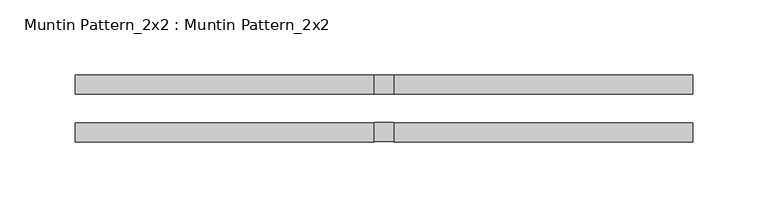
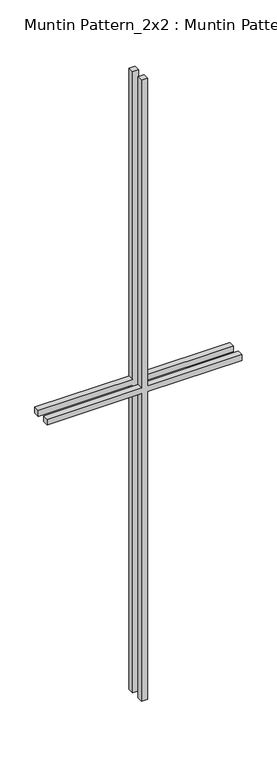
"""IFC4 building model written with IfcOpenShell, lengths in millimetres: proxy geometry, Muntin Pattern_2x2 : Muntin Pattern_2x2."""

from ifc_helpers import new_model, si_unit, frame, origin, place, context, project, spatial, polyline, outline, extrude, source, transform, mapped, element, save


def muntin_pattern_2x2_muntin_pattern_2x2_63bd3b25(model_context):
    return source(origin(), model_context, "Body", "SweptSolid", [
        extrude(outline(polyline([(698.5, -6.35), (698.5, -205.5885801), (685.8, -205.5885801), (685.8, -6.35), (0.0, -6.35), (0.0, 6.35), (685.8, 6.35), (685.8, 205.5885801), (698.5, 205.5885801), (698.5, 6.35), (1384.3, 6.35), (1384.3, -6.35), (698.5, -6.35)])), frame((0.0, 9.525, 0.0), z_axis=(0.0, 1.0, 0.0), x_axis=(0.0, 0.0, 1.0)), (0.0, 0.0, 1.0), 12.7),
        extrude(outline(polyline([(698.5, -6.35), (698.5, -205.5885801), (685.8, -205.5885801), (685.8, -6.35), (0.0, -6.35), (0.0, 6.35), (685.8, 6.35), (685.8, 205.5885801), (698.5, 205.5885801), (698.5, 6.35), (1384.3, 6.35), (1384.3, -6.35), (698.5, -6.35)])), frame((0.0, -22.225, 0.0), z_axis=(0.0, 1.0, 0.0), x_axis=(0.0, 0.0, 1.0)), (0.0, 0.0, 1.0), 12.7),
    ])


if __name__ == "__main__":
    model = new_model("IFC4")
    model_context = context("Model", 3, world=origin())
    ifc_project = project(units=[si_unit("LENGTHUNIT", "METRE", prefix="MILLI")], contexts=[model_context])
    site = spatial("IfcSite", under=ifc_project)
    building = spatial("IfcBuilding", under=site)
    placement = place(None, origin())
    muntin_pattern_2x2_muntin_pattern_2x2_shape = muntin_pattern_2x2_muntin_pattern_2x2_63bd3b25(model_context)
    element("IfcBuildingElementProxy", 1, Name="Muntin Pattern_2x2 : Muntin Pattern_2x2", ObjectType="Muntin Pattern_2x2 : Muntin Pattern_2x2", at=placement, inside=building, context=model_context, shape_type="MappedRepresentation", body=[
        mapped(muntin_pattern_2x2_muntin_pattern_2x2_shape, transform((0.0, 0.0, 0.0), x_axis=(1.0, 0.0, 0.0), y_axis=(0.0, 1.0, 0.0), z_axis=(0.0, 0.0, 1.0))),
    ])
    save(model, "model.ifc")

# Revit data of these elements
# Type "Muntin Pattern_2x2 : Muntin Pattern_2x2"
#   Width [instance default] = 4' - 0"
#   Thickness = 0' - 0 1/2"
#   Height [instance default] = 4' - 0"
#   Distance = 0' - 0 3/4"
#   Interior Material [instance default] = none
#   Exterior Material [instance default] = none
#   Default Elevation = 0
# Element 1 (IfcBuildingElementProxy, "Muntin Pattern_2x2 : Muntin Pattern_2x2")
#   Width = 1' - 4.18808"
#   Height = 4' - 6 1/2"
#   Interior Material = Wood - Stained
#   Exterior Material = Clad - White
#   Materials on its faces: "Clad - White", "Wood - Stained"
# Materials
#   "Clad - White": class "Wood", colour RGB 242 242 238, transparency 0, Cost = 0
#   "Wood - Stained": class "Wood", colour RGB 227 170 128, transparency 0, Cost = 0
